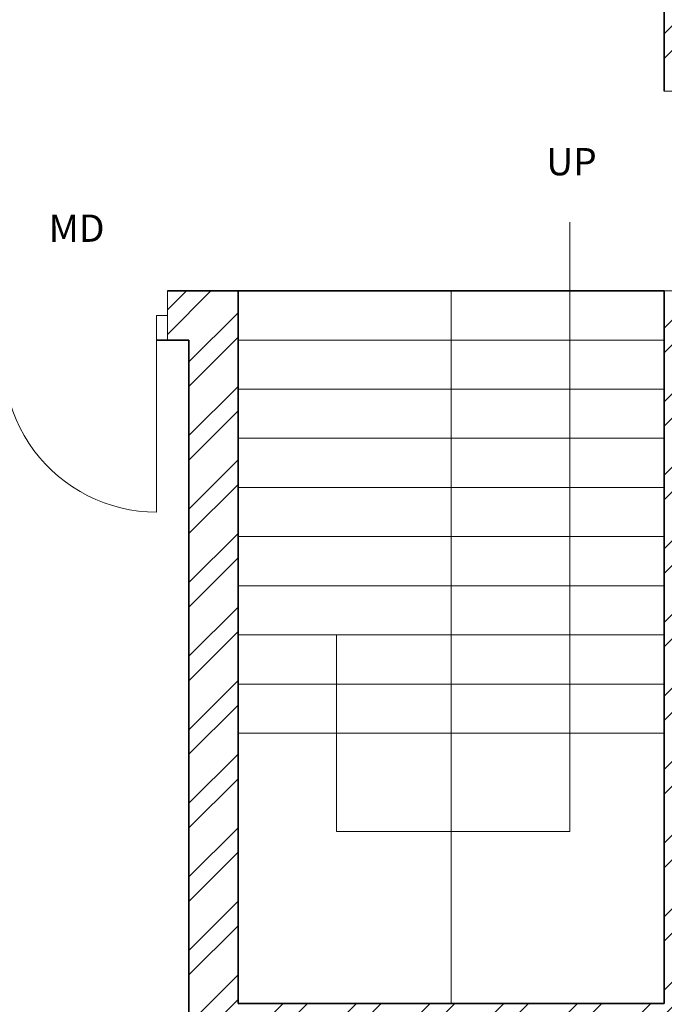
# Model space of a CAD drawing. Units: inches. Extents: x 2120 to 4013, y 1390 to 3019.
# Tile 15 of 59: x 2598 to 2716, y 1784 to 1964. Entities that reach past the tile are written whole.
import ezdxf

# ---------------------------------------------------------------- set-up
doc = ezdxf.new("R2010")
doc.units = ezdxf.units.IN
for name, color, linetype, lineweight in [('A-ANNO-TEXT', 7, 'Continuous', 18), ('A-DOOR', 3, 'Continuous', 18), ('A-FLOR-STRS', 7, 'Continuous', 18), ('A-WALL', 7, 'Continuous', 35), ('A-WALL-PATT', 252, 'Continuous', 13)]:
    doc.layers.add(name, color=color, linetype=linetype, lineweight=lineweight)
doc.styles.get("Standard").update_dxf_attribs({"font": 'arial.ttf'})

# ---------------------------------------------------------------- blocks, each defined once
blk = doc.blocks.new('DOOR-SWING-36IN-109p07DEG')
for p, q in [((9, 36.56), (0, 36.56)), ((0, 36.56), (4.5, 36.56)), ((4.5, 36.56), (4.5, 34.56)), ((9, 36.56), (9, 36.56)), ((4.5, 34.56), (40.5, 34.56)), ((4.5, 0), (4.5, 2)), ((9, 0), (0, 0)), ((0, 0), (4.5, 0))]:
    blk.add_line(p, q)
blk.add_arc((10.9, 31.1), 29.8, 257.5927, 6.6652)
blk = doc.blocks.new('DOOR-SWING-36IN-106p79DEG')
for p, q in [((0, 40.5), (0, 31.5)), ((30.74, 31.5), (30.74, 40.5)), ((30.74, 40.5), (30.74, 36)), ((0, 31.5), (0, 36)), ((0, 36), (2, 36)), ((30.74, 36), (28.74, 36)), ((28.74, 36), (28.74, 0))]:
    blk.add_line(p, q)
blk.add_arc((28.74, 27.93), 27.93, 163.2075, 270)
blk = doc.blocks.new('STAIR-DOGLEG-PLAN')
for p, q in [((60.72, 143.1), (60.72, 31.5)), ((39, 0), (39, 130.5)), ((78, 121.5), (0, 121.5)), ((78, 112.5), (0, 112.5)), ((78, 103.5), (0, 103.5)), ((78, 94.5), (0, 94.5)), ((78, 85.5), (0, 85.5)), ((78, 76.5), (0, 76.5)), ((78, 67.5), (0, 67.5)), ((18.01, 31.5), (18.01, 67.5)), ((78, 58.5), (0, 58.5)), ((78, 49.5), (0, 49.5)), ((60.72, 31.5), (18.01, 31.5)), ((60.72, 31.5), (18.01, 31.5))]:
    blk.add_line(p, q)

msp = doc.modelspace()

# ---------------------------------------------------------------- hatches: boundary and pattern name
at = {"layer": 'A-WALL-PATT'}
h = msp.add_hatch(dxfattribs=at)
h.set_pattern_fill('ANSI32', color=256)
h.paths.add_polyline_path([(2271.7331, 2343.531), (2283.3788, 2343.531), (2283.3788, 2348.031), (2283.3788, 2352.5306), (2262.7331, 2352.5306), (2262.7331, 2182.638), (2267.2331, 2182.638), (2271.7331, 2182.638), (2271.7331, 2219.031), (2391.7331, 2219.031), (2391.7331, 2214.189), (2393.9831, 2214.189), (2396.2331, 2214.189), (2396.2331, 2219.031), (2420.2331, 2219.031), (2420.2331, 2225.7535), (2417.2197, 2225.7535), (2415.7331, 2225.7535), (2415.7331, 2223.5306), (2271.7331, 2223.5306)])
h.paths.add_polyline_path([(2380.0942, 2352.5306), (2343.3788, 2352.5306), (2343.3788, 2343.531), (2363.2331, 2343.531), (2363.2331, 2288.8489), (2365.4831, 2288.8489), (2367.7331, 2288.8489), (2367.7331, 2343.531), (2380.0942, 2343.531)], flags=17)
h.paths.add_polyline_path([(2432.4339, 2352.5306), (2404.0943, 2352.5306), (2404.0943, 2343.531), (2415.7331, 2343.531), (2415.7331, 2264.0306), (2367.7331, 2264.0306), (2367.7331, 2266.4872), (2363.2331, 2266.4872), (2363.2331, 2259.531), (2367.7331, 2259.531), (2415.7331, 2259.531), (2415.7331, 2255.0658), (2420.2331, 2255.0658), (2420.2331, 2259.531), (2424.5717, 2259.531), (2424.5717, 2261.781), (2424.5717, 2264.0306), (2420.2331, 2264.0306), (2420.2331, 2343.531), (2432.4339, 2343.531)])
h.paths.add_polyline_path([(2508.9115, 2352.5306), (2456.4339, 2352.5306), (2456.4339, 2343.531), (2468.2331, 2343.531), (2468.2331, 2264.0306), (2448.0487, 2264.0306), (2448.0487, 2259.531), (2468.2331, 2259.531), (2468.2331, 2255.5496), (2472.7331, 2255.5496), (2472.7331, 2343.531), (2508.9115, 2343.531)])
h.paths.add_polyline_path([(2637.7331, 2352.5306), (2544.9116, 2352.5306), (2544.9116, 2343.531), (2589.7331, 2343.531), (2633.2331, 2343.531), (2637.7331, 2343.531)])
h.paths.add_polyline_path([(2594.2331, 2343.5306), (2589.7331, 2343.5306), (2589.7331, 2259.5306), (2589.7331, 2252.4915), (2591.9831, 2252.4915), (2594.2331, 2252.4915)])
h.paths.add_polyline_path([(2637.7331, 2223.5306), (2594.2331, 2223.5306), (2594.2331, 2230.1988), (2591.9831, 2230.1988), (2589.7331, 2230.1988), (2589.7331, 2223.5306), (2472.7331, 2223.5306), (2468.2331, 2223.5306), (2468.2331, 2219.031), (2628.7331, 2219.031), (2628.7331, 2138.031), (2637.7331, 2138.031)])
h.paths.add_polyline_path([(3822.6535, 2458.4402), (3874.9468, 2458.4402), (3874.9468, 2476.9866), (3822.6535, 2476.9866)], flags=9)
h.paths.add_polyline_path([(3834.6921, 2781.8174), (3935.9206, 2781.8174), (3935.9206, 2800.3638), (3834.6921, 2800.3638)], flags=9)
h.paths.add_polyline_path([(3832.2843, 2837.9683), (3884.5776, 2837.9683), (3884.5776, 2856.5146), (3832.2843, 2856.5146)], flags=9)
h.paths.add_polyline_path([(3830.9388, 2861.4782), (3956.8958, 2861.4782), (3956.8958, 2880.0245), (3830.9388, 2880.0245)], flags=9)
h.paths.add_polyline_path([(3870.6966, 2352.5752), (3887.9272, 2352.5752), (3887.9272, 2377.3037), (3870.6966, 2377.3037)], flags=9)
h.paths.add_polyline_path([(3289.2701, 2413.161), (3435.2223, 2413.161), (3435.2223, 2450.2538), (3289.2701, 2450.2538)], flags=9)
h.paths.add_polyline_path([(2487.6944, 2414.3601), (2637.8335, 2414.3601), (2637.8335, 2451.4528), (2487.6944, 2451.4528)], flags=9)
h.paths.add_polyline_path([(2567.3724, 1457.9199), (2815.296, 1457.9199), (2815.296, 1495.0127), (2567.3724, 1495.0127)], flags=9)
h.paths.add_polyline_path([(2655.3825, 2093.2363), (2685.9555, 2093.2363), (2685.9555, 2111.8937), (2655.3825, 2111.8937)], flags=9)
h.paths.add_polyline_path([(2543.9218, 1550.6671), (2587.8406, 1550.6671), (2587.8406, 1569.3244), (2543.9218, 1569.3244)], flags=9)
h.paths.add_polyline_path([(2905.1384, 1543.8113), (2949.0572, 1543.8113), (2949.0572, 1562.4686), (2905.1384, 1562.4686)], flags=9)
h.paths.add_polyline_path([(2736.4118, 1702.4736), (2784.2153, 1702.4736), (2784.2153, 1721.1309), (2736.4118, 1721.1309)], flags=9)
h.paths.add_polyline_path([(2912.8666, 1710.4168), (2951.707, 1710.4168), (2951.707, 1729.0741), (2912.8666, 1729.0741)], flags=9)
h.paths.add_polyline_path([(2923.5785, 1763.5038), (2959.7279, 1763.5038), (2959.7279, 1782.1611), (2923.5785, 1782.1611)], flags=9)
h.paths.add_polyline_path([(2925.2114, 1809.6137), (2967.1861, 1809.6137), (2967.1861, 1828.271), (2925.2114, 1828.271)], flags=9)
h.paths.add_polyline_path([(2996.2711, 1878.9003), (2996.2711, 1913.109), (2977.6138, 1913.109), (2977.6138, 1878.9003)], flags=9)
h.paths.add_polyline_path([(2883.0859, 1895.7192), (2927.1855, 1895.7192), (2927.1855, 1914.3766), (2883.0859, 1914.3766)], flags=9)
h.paths.add_polyline_path([(2787.3924, 1810.8013), (2841.0213, 1810.8013), (2841.0213, 1829.4587), (2787.3924, 1829.4587)], flags=9)
h.paths.add_polyline_path([(2775.6399, 2101.7395), (2829.2689, 2101.7395), (2829.2689, 2120.3968), (2775.6399, 2120.3968)], flags=9)
h.paths.add_polyline_path([(2913.0263, 2075.817), (2951.8667, 2075.817), (2951.8667, 2094.4744), (2913.0263, 2094.4744)], flags=9)
h.paths.add_polyline_path([(2929.966, 2133.3669), (2966.1154, 2133.3669), (2966.1154, 2152.0243), (2929.966, 2152.0243)], flags=9)
h.paths.add_polyline_path([(2932.7502, 2182.6088), (2968.8996, 2182.6088), (2968.8996, 2201.2662), (2932.7502, 2201.2662)], flags=9)
h.paths.add_polyline_path([(2996.0681, 2266.3173), (2996.0681, 2300.5261), (2977.4108, 2300.5261), (2977.4108, 2266.3173)], flags=9)
h.paths.add_polyline_path([(2885.1039, 2279.2186), (2929.2035, 2279.2186), (2929.2035, 2297.8759), (2885.1039, 2297.8759)], flags=9)
h.paths.add_polyline_path([(2735.7042, 2218.3197), (2783.5078, 2218.3197), (2783.5078, 2236.9771), (2735.7042, 2236.9771)], flags=9)
h.paths.add_polyline_path([(2635.6049, 2044.0085), (2648.9678, 2044.0085), (2648.9678, 2054.312), (2635.6049, 2054.312)], flags=9)
h.paths.add_polyline_path([(2714.0148, 1923.0473), (2727.3777, 1923.0473), (2727.3777, 1933.3508), (2714.0148, 1933.3508)], flags=9)
h.paths.add_polyline_path([(2709.0345, 1988.1628), (2722.3974, 1988.1628), (2722.3974, 1998.4663), (2709.0345, 1998.4663)], flags=9)
h.paths.add_polyline_path([(2592.8935, 1962.1763), (2606.2564, 1962.1763), (2606.2564, 1972.4799), (2592.8935, 1972.4799)], flags=9)
h.paths.add_polyline_path([(2618.3996, 1985.9724), (2644.1942, 1985.9724), (2644.1942, 1996.2759), (2618.3996, 1996.2759)], flags=9)
h.paths.add_polyline_path([(2601.279, 1920.5869), (2614.6419, 1920.5869), (2614.6419, 1930.8904), (2601.279, 1930.8904)], flags=9)
h.paths.add_polyline_path([(2692.3278, 1932.7645), (2704.5311, 1932.7645), (2704.5311, 1943.0681), (2692.3278, 1943.0681)], flags=9)
h.paths.add_polyline_path([(2311.122, 1672.7318), (2355.0408, 1672.7318), (2355.0408, 1691.3892), (2311.122, 1691.3892)], flags=9)
h.paths.add_polyline_path([(2456.2551, 1632.3198), (2492.4796, 1632.3198), (2492.4796, 1650.9772), (2456.2551, 1650.9772)], flags=9)
h.paths.add_polyline_path([(2401.0766, 1631.4793), (2437.301, 1631.4793), (2437.301, 1650.1367), (2401.0766, 1650.1367)], flags=9)
h.paths.add_polyline_path([(2546.7054, 1700.9235), (2594.509, 1700.9235), (2594.509, 1719.5809), (2546.7054, 1719.5809)], flags=9)
h.paths.add_polyline_path([(2445.4866, 1766.9937), (2497.5261, 1766.9937), (2497.5261, 1785.651), (2445.4866, 1785.651)], flags=9)
h.paths.add_polyline_path([(2287.9992, 1739.7675), (2326.8396, 1739.7675), (2326.8396, 1758.4248), (2287.9992, 1758.4248)], flags=9)
h.paths.add_polyline_path([(2458.5279, 1924.7607), (2510.5675, 1924.7607), (2510.5675, 1943.4181), (2458.5279, 1943.4181)], flags=9)
h.paths.add_polyline_path([(2309.2811, 1902.7642), (2345.4305, 1902.7642), (2345.4305, 1921.4215), (2309.2811, 1921.4215)], flags=9)
h.paths.add_polyline_path([(2490.7554, 2018.9392), (2530.7896, 2018.9392), (2530.7896, 2037.5965), (2490.7554, 2037.5965)], flags=9)
h.paths.add_polyline_path([(2402.143, 2024.7393), (2438.5414, 2024.7393), (2438.5414, 2043.3966), (2402.143, 2043.3966)], flags=9)
h.paths.add_polyline_path([(2287.856, 1931.7926), (2326.6964, 1931.7926), (2326.6964, 1950.4499), (2287.856, 1950.4499)], flags=9)
h.paths.add_polyline_path([(2281.7979, 2193.5771), (2320.6383, 2193.5771), (2320.6383, 2212.2344), (2281.7979, 2212.2344)], flags=25)
h.paths.add_polyline_path([(2484.0754, 2093.892), (2536.115, 2093.892), (2536.115, 2112.5494), (2484.0754, 2112.5494)], flags=9)
h.paths.add_polyline_path([(2624.7948, 2281.8639), (2624.7948, 2311.4137), (2606.1375, 2311.4137), (2606.1375, 2281.8639)], flags=9)
h.paths.add_polyline_path([(2507.5036, 2290.3639), (2541.934, 2290.3639), (2541.934, 2309.0212), (2507.5036, 2309.0212)], flags=9)
h.paths.add_polyline_path([(2423.1076, 2285.2202), (2459.332, 2285.2202), (2459.332, 2303.8776), (2423.1076, 2303.8776)], flags=9)
h.paths.add_polyline_path([(2374.5467, 2289.6272), (2410.7711, 2289.6272), (2410.7711, 2308.2846), (2374.5467, 2308.2846)], flags=25)
h.paths.add_polyline_path([(2277.4907, 2227.5651), (2316.3311, 2227.5651), (2316.3311, 2246.2224), (2277.4907, 2246.2224)], flags=25)
h.paths.add_polyline_path([(2655.3825, 2093.2367), (2685.9555, 2093.2367), (2685.9555, 2111.894), (2655.3825, 2111.894)], flags=9)
h.paths.add_polyline_path([(2543.9217, 1550.6674), (2587.8406, 1550.6674), (2587.8406, 1569.3247), (2543.9217, 1569.3247)], flags=9)
h.paths.add_polyline_path([(2905.1384, 1543.8116), (2949.0572, 1543.8116), (2949.0572, 1562.4689), (2905.1384, 1562.4689)], flags=9)
h.paths.add_polyline_path([(2736.4118, 1702.4739), (2784.2153, 1702.4739), (2784.2153, 1721.1312), (2736.4118, 1721.1312)], flags=9)
h.paths.add_polyline_path([(2912.8666, 1710.4171), (2951.707, 1710.4171), (2951.707, 1729.0744), (2912.8666, 1729.0744)], flags=9)
h.paths.add_polyline_path([(2923.5785, 1763.5041), (2959.7279, 1763.5041), (2959.7279, 1782.1614), (2923.5785, 1782.1614)], flags=9)
h.paths.add_polyline_path([(2925.2114, 1809.614), (2967.1861, 1809.614), (2967.1861, 1828.2713), (2925.2114, 1828.2713)], flags=9)
h.paths.add_polyline_path([(2996.2711, 1878.9006), (2996.2711, 1913.1094), (2977.6137, 1913.1094), (2977.6137, 1878.9006)], flags=9)
h.paths.add_polyline_path([(2883.0859, 1895.7195), (2927.1855, 1895.7195), (2927.1855, 1914.3769), (2883.0859, 1914.3769)], flags=9)
h.paths.add_polyline_path([(2787.3924, 1810.8016), (2841.0213, 1810.8016), (2841.0213, 1829.459), (2787.3924, 1829.459)], flags=9)
h.paths.add_polyline_path([(2775.6399, 2101.7398), (2829.2688, 2101.7398), (2829.2688, 2120.3971), (2775.6399, 2120.3971)], flags=9)
h.paths.add_polyline_path([(2913.0263, 2075.8173), (2951.8667, 2075.8173), (2951.8667, 2094.4747), (2913.0263, 2094.4747)], flags=9)
h.paths.add_polyline_path([(2929.966, 2133.3672), (2966.1154, 2133.3672), (2966.1154, 2152.0246), (2929.966, 2152.0246)], flags=9)
h.paths.add_polyline_path([(2932.7502, 2182.6091), (2968.8996, 2182.6091), (2968.8996, 2201.2665), (2932.7502, 2201.2665)], flags=9)
h.paths.add_polyline_path([(2996.0681, 2266.3176), (2996.0681, 2300.5264), (2977.4108, 2300.5264), (2977.4108, 2266.3176)], flags=9)
h.paths.add_polyline_path([(2885.1039, 2279.2189), (2929.2035, 2279.2189), (2929.2035, 2297.8762), (2885.1039, 2297.8762)], flags=9)
h.paths.add_polyline_path([(2735.7042, 2218.32), (2783.5078, 2218.32), (2783.5078, 2236.9774), (2735.7042, 2236.9774)], flags=9)
h.paths.add_polyline_path([(2635.6048, 2044.0088), (2648.9677, 2044.0088), (2648.9677, 2054.3123), (2635.6048, 2054.3123)], flags=9)
h.paths.add_polyline_path([(2714.0148, 1923.0476), (2727.3777, 1923.0476), (2727.3777, 1933.3511), (2714.0148, 1933.3511)], flags=9)
h.paths.add_polyline_path([(2709.0345, 1988.1631), (2722.3974, 1988.1631), (2722.3974, 1998.4666), (2709.0345, 1998.4666)], flags=9)
h.paths.add_polyline_path([(2592.8935, 1962.1766), (2606.2564, 1962.1766), (2606.2564, 1972.4802), (2592.8935, 1972.4802)], flags=9)
h.paths.add_polyline_path([(2618.3995, 1985.9727), (2644.1942, 1985.9727), (2644.1942, 1996.2762), (2618.3995, 1996.2762)], flags=9)
h.paths.add_polyline_path([(2601.279, 1920.5872), (2614.6419, 1920.5872), (2614.6419, 1930.8908), (2601.279, 1930.8908)], flags=9)
h.paths.add_polyline_path([(2692.3278, 1932.7648), (2704.5311, 1932.7648), (2704.5311, 1943.0684), (2692.3278, 1943.0684)], flags=9)
h.paths.add_polyline_path([(2311.122, 1672.7321), (2355.0408, 1672.7321), (2355.0408, 1691.3895), (2311.122, 1691.3895)], flags=9)
h.paths.add_polyline_path([(2456.2551, 1632.3201), (2492.4795, 1632.3201), (2492.4795, 1650.9775), (2456.2551, 1650.9775)], flags=9)
h.paths.add_polyline_path([(2401.0766, 1631.4796), (2437.301, 1631.4796), (2437.301, 1650.137), (2401.0766, 1650.137)], flags=9)
h.paths.add_polyline_path([(2546.7054, 1700.9238), (2594.509, 1700.9238), (2594.509, 1719.5812), (2546.7054, 1719.5812)], flags=9)
h.paths.add_polyline_path([(2445.4866, 1766.994), (2497.5261, 1766.994), (2497.5261, 1785.6513), (2445.4866, 1785.6513)], flags=9)
h.paths.add_polyline_path([(2287.9992, 1739.7678), (2326.8396, 1739.7678), (2326.8396, 1758.4251), (2287.9992, 1758.4251)], flags=9)
h.paths.add_polyline_path([(2458.5279, 1924.7611), (2510.5675, 1924.7611), (2510.5675, 1943.4184), (2458.5279, 1943.4184)], flags=9)
h.paths.add_polyline_path([(2309.2811, 1902.7645), (2345.4305, 1902.7645), (2345.4305, 1921.4218), (2309.2811, 1921.4218)], flags=9)
h.paths.add_polyline_path([(2490.7554, 2018.9395), (2530.7895, 2018.9395), (2530.7895, 2037.5968), (2490.7554, 2037.5968)], flags=9)
h.paths.add_polyline_path([(2402.143, 2024.7396), (2438.5413, 2024.7396), (2438.5413, 2043.3969), (2402.143, 2043.3969)], flags=9)
h.paths.add_polyline_path([(2287.856, 1931.7929), (2326.6964, 1931.7929), (2326.6964, 1950.4502), (2287.856, 1950.4502)], flags=9)
h.paths.add_polyline_path([(2281.7979, 2193.5774), (2320.6383, 2193.5774), (2320.6383, 2212.2347), (2281.7979, 2212.2347)], flags=25)
h.paths.add_polyline_path([(2484.0754, 2093.8924), (2536.115, 2093.8924), (2536.115, 2112.5497), (2484.0754, 2112.5497)], flags=9)
h.paths.add_polyline_path([(2624.7948, 2281.8642), (2624.7948, 2311.414), (2606.1374, 2311.414), (2606.1374, 2281.8642)], flags=9)
h.paths.add_polyline_path([(2507.5035, 2290.3642), (2541.934, 2290.3642), (2541.934, 2309.0215), (2507.5035, 2309.0215)], flags=9)
h.paths.add_polyline_path([(2423.1075, 2285.2205), (2459.332, 2285.2205), (2459.332, 2303.8779), (2423.1075, 2303.8779)], flags=9)
h.paths.add_polyline_path([(2374.5467, 2289.6275), (2410.7711, 2289.6275), (2410.7711, 2308.2849), (2374.5467, 2308.2849)], flags=25)
h.paths.add_polyline_path([(2277.4907, 2227.5654), (2316.3311, 2227.5654), (2316.3311, 2246.2227), (2277.4907, 2246.2227)], flags=25)
h = msp.add_hatch(dxfattribs=at)
h.set_pattern_fill('ANSI32', color=256)
h.paths.add_polyline_path([(2271.7331, 1980.389), (2262.7331, 1980.389), (2262.7331, 1912.8434), (2267.2331, 1912.8434), (2271.7331, 1912.8434), (2271.7331, 1922.531), (2351.2331, 1922.531), (2351.2331, 1901.4728), (2355.7331, 1901.4728), (2355.7331, 1922.531), (2357.9815, 1922.531), (2357.9815, 1926.5306), (2271.7331, 1926.5306)])
h.paths.add_polyline_path([(2589.2331, 1949.1622), (2584.7331, 1949.1622), (2580.2331, 1949.1622), (2580.2331, 1874.5306), (2355.7331, 1874.5306), (2355.7331, 1880.1922), (2351.2331, 1880.1922), (2351.2331, 1874.5306), (2271.7331, 1874.5306), (2271.7331, 1888.8431), (2262.7331, 1888.8431), (2262.7331, 1842.2909), (2267.2331, 1842.2909), (2271.7331, 1842.2909), (2271.7331, 1865.531), (2415.7331, 1865.531), (2415.7331, 1779.7286), (2420.2331, 1779.7286), (2420.2331, 1865.531), (2589.2331, 1865.531)])
h.paths.add_polyline_path([(2271.7331, 1782.2906), (2262.7331, 1782.2906), (2262.7331, 1711.4639), (2267.2331, 1711.4639), (2271.7331, 1711.4639), (2271.7331, 1738.031), (2420.2331, 1738.031), (2420.2331, 1742.531), (2420.2331, 1747.3376), (2417.9831, 1747.3376), (2415.7331, 1747.3376), (2415.7331, 1742.5306), (2271.7331, 1742.5306)])
h.paths.add_polyline_path([(2271.7331, 1627.031), (2362.3957, 1627.031), (2362.3957, 1629.281), (2362.3957, 1631.5306), (2271.7331, 1631.5306), (2271.7331, 1675.4636), (2262.7331, 1675.4636), (2262.7331, 1581.531), (2405.3032, 1581.531), (2405.3032, 1586.031), (2405.3032, 1590.5306), (2396.2331, 1590.5306), (2396.2331, 1691.4513), (2418.7206, 1691.4513), (2418.7206, 1695.951), (2396.2331, 1695.951), (2391.7331, 1695.951), (2391.7331, 1631.5306), (2386.7425, 1631.5306), (2386.7425, 1629.2806), (2386.7425, 1627.031), (2391.7331, 1627.031), (2391.7331, 1586.1709), (2271.7331, 1586.1709)])
h.paths.add_polyline_path([(2459.6703, 1590.5306), (2429.3032, 1590.5306), (2429.3032, 1581.531), (2459.6703, 1581.531), (2459.6703, 1586.031)])
h.paths.add_polyline_path([(2501.2331, 1590.531), (2501.2331, 1665.0195), (2498.9831, 1665.0195), (2496.7331, 1665.0195), (2496.7331, 1590.5306), (2483.8201, 1590.5306), (2483.8201, 1590.1579), (2483.6704, 1590.1579), (2483.6704, 1581.531), (2505.0196, 1581.531), (2505.0196, 1583.781), (2505.0196, 1586.0306), (2501.2331, 1586.0306)])
h.paths.add_polyline_path([(2544.1361, 1583.781), (2544.1361, 1586.0306), (2527.1368, 1586.0306), (2527.1368, 1583.7806), (2527.1368, 1581.531), (2544.1361, 1581.531)])
h.paths.add_polyline_path([(3822.6535, 2458.4402), (3874.9468, 2458.4402), (3874.9468, 2476.9866), (3822.6535, 2476.9866)], flags=9)
h.paths.add_polyline_path([(3834.6921, 2781.8174), (3935.9206, 2781.8174), (3935.9206, 2800.3638), (3834.6921, 2800.3638)], flags=9)
h.paths.add_polyline_path([(3832.2843, 2837.9683), (3884.5776, 2837.9683), (3884.5776, 2856.5146), (3832.2843, 2856.5146)], flags=9)
h.paths.add_polyline_path([(3830.9388, 2861.4782), (3956.8958, 2861.4782), (3956.8958, 2880.0245), (3830.9388, 2880.0245)], flags=9)
h.paths.add_polyline_path([(3870.6966, 2352.5752), (3887.9272, 2352.5752), (3887.9272, 2377.3037), (3870.6966, 2377.3037)], flags=9)
h.paths.add_polyline_path([(3289.2701, 2413.161), (3435.2223, 2413.161), (3435.2223, 2450.2538), (3289.2701, 2450.2538)], flags=9)
h.paths.add_polyline_path([(2487.6944, 2414.3601), (2637.8335, 2414.3601), (2637.8335, 2451.4528), (2487.6944, 2451.4528)], flags=9)
h.paths.add_polyline_path([(2567.3724, 1457.9199), (2815.296, 1457.9199), (2815.296, 1495.0127), (2567.3724, 1495.0127)], flags=9)
h.paths.add_polyline_path([(2655.3825, 2093.2363), (2685.9555, 2093.2363), (2685.9555, 2111.8937), (2655.3825, 2111.8937)], flags=9)
h.paths.add_polyline_path([(2543.9218, 1550.6671), (2587.8406, 1550.6671), (2587.8406, 1569.3244), (2543.9218, 1569.3244)], flags=9)
h.paths.add_polyline_path([(2905.1384, 1543.8113), (2949.0572, 1543.8113), (2949.0572, 1562.4686), (2905.1384, 1562.4686)], flags=9)
h.paths.add_polyline_path([(2736.4118, 1702.4736), (2784.2153, 1702.4736), (2784.2153, 1721.1309), (2736.4118, 1721.1309)], flags=9)
h.paths.add_polyline_path([(2912.8666, 1710.4168), (2951.707, 1710.4168), (2951.707, 1729.0741), (2912.8666, 1729.0741)], flags=9)
h.paths.add_polyline_path([(2923.5785, 1763.5038), (2959.7279, 1763.5038), (2959.7279, 1782.1611), (2923.5785, 1782.1611)], flags=9)
h.paths.add_polyline_path([(2925.2114, 1809.6137), (2967.1861, 1809.6137), (2967.1861, 1828.271), (2925.2114, 1828.271)], flags=9)
h.paths.add_polyline_path([(2996.2711, 1878.9003), (2996.2711, 1913.109), (2977.6138, 1913.109), (2977.6138, 1878.9003)], flags=9)
h.paths.add_polyline_path([(2883.0859, 1895.7192), (2927.1855, 1895.7192), (2927.1855, 1914.3766), (2883.0859, 1914.3766)], flags=9)
h.paths.add_polyline_path([(2787.3924, 1810.8013), (2841.0213, 1810.8013), (2841.0213, 1829.4587), (2787.3924, 1829.4587)], flags=9)
h.paths.add_polyline_path([(2775.6399, 2101.7395), (2829.2689, 2101.7395), (2829.2689, 2120.3968), (2775.6399, 2120.3968)], flags=9)
h.paths.add_polyline_path([(2913.0263, 2075.817), (2951.8667, 2075.817), (2951.8667, 2094.4744), (2913.0263, 2094.4744)], flags=9)
h.paths.add_polyline_path([(2929.966, 2133.3669), (2966.1154, 2133.3669), (2966.1154, 2152.0243), (2929.966, 2152.0243)], flags=9)
h.paths.add_polyline_path([(2932.7502, 2182.6088), (2968.8996, 2182.6088), (2968.8996, 2201.2662), (2932.7502, 2201.2662)], flags=9)
h.paths.add_polyline_path([(2996.0681, 2266.3173), (2996.0681, 2300.5261), (2977.4108, 2300.5261), (2977.4108, 2266.3173)], flags=9)
h.paths.add_polyline_path([(2885.1039, 2279.2186), (2929.2035, 2279.2186), (2929.2035, 2297.8759), (2885.1039, 2297.8759)], flags=9)
h.paths.add_polyline_path([(2735.7042, 2218.3197), (2783.5078, 2218.3197), (2783.5078, 2236.9771), (2735.7042, 2236.9771)], flags=9)
h.paths.add_polyline_path([(2635.6049, 2044.0085), (2648.9678, 2044.0085), (2648.9678, 2054.312), (2635.6049, 2054.312)], flags=9)
h.paths.add_polyline_path([(2714.0148, 1923.0473), (2727.3777, 1923.0473), (2727.3777, 1933.3508), (2714.0148, 1933.3508)], flags=9)
h.paths.add_polyline_path([(2709.0345, 1988.1628), (2722.3974, 1988.1628), (2722.3974, 1998.4663), (2709.0345, 1998.4663)], flags=9)
h.paths.add_polyline_path([(2592.8935, 1962.1763), (2606.2564, 1962.1763), (2606.2564, 1972.4799), (2592.8935, 1972.4799)], flags=9)
h.paths.add_polyline_path([(2618.3996, 1985.9724), (2644.1942, 1985.9724), (2644.1942, 1996.2759), (2618.3996, 1996.2759)], flags=9)
h.paths.add_polyline_path([(2601.279, 1920.5869), (2614.6419, 1920.5869), (2614.6419, 1930.8904), (2601.279, 1930.8904)], flags=9)
h.paths.add_polyline_path([(2692.3278, 1932.7645), (2704.5311, 1932.7645), (2704.5311, 1943.0681), (2692.3278, 1943.0681)], flags=9)
h.paths.add_polyline_path([(2311.122, 1672.7318), (2355.0408, 1672.7318), (2355.0408, 1691.3892), (2311.122, 1691.3892)], flags=25)
h.paths.add_polyline_path([(2456.2551, 1632.3198), (2492.4796, 1632.3198), (2492.4796, 1650.9772), (2456.2551, 1650.9772)], flags=9)
h.paths.add_polyline_path([(2401.0766, 1631.4793), (2437.301, 1631.4793), (2437.301, 1650.1367), (2401.0766, 1650.1367)], flags=9)
h.paths.add_polyline_path([(2546.7054, 1700.9235), (2594.509, 1700.9235), (2594.509, 1719.5809), (2546.7054, 1719.5809)], flags=9)
h.paths.add_polyline_path([(2445.4866, 1766.9937), (2497.5261, 1766.9937), (2497.5261, 1785.651), (2445.4866, 1785.651)], flags=9)
h.paths.add_polyline_path([(2287.9992, 1739.7675), (2326.8396, 1739.7675), (2326.8396, 1758.4248), (2287.9992, 1758.4248)], flags=24)
h.paths.add_polyline_path([(2458.5279, 1924.7607), (2510.5675, 1924.7607), (2510.5675, 1943.4181), (2458.5279, 1943.4181)], flags=25)
h.paths.add_polyline_path([(2309.2811, 1902.7642), (2345.4305, 1902.7642), (2345.4305, 1921.4215), (2309.2811, 1921.4215)], flags=25)
h.paths.add_polyline_path([(2490.7554, 2018.9392), (2530.7896, 2018.9392), (2530.7896, 2037.5965), (2490.7554, 2037.5965)], flags=9)
h.paths.add_polyline_path([(2402.143, 2024.7393), (2438.5414, 2024.7393), (2438.5414, 2043.3966), (2402.143, 2043.3966)], flags=9)
h.paths.add_polyline_path([(2287.856, 1931.7926), (2326.6964, 1931.7926), (2326.6964, 1950.4499), (2287.856, 1950.4499)], flags=25)
h.paths.add_polyline_path([(2281.7979, 2193.5771), (2320.6383, 2193.5771), (2320.6383, 2212.2344), (2281.7979, 2212.2344)], flags=9)
h.paths.add_polyline_path([(2484.0754, 2093.892), (2536.115, 2093.892), (2536.115, 2112.5494), (2484.0754, 2112.5494)], flags=9)
h.paths.add_polyline_path([(2624.7948, 2281.8639), (2624.7948, 2311.4137), (2606.1375, 2311.4137), (2606.1375, 2281.8639)], flags=9)
h.paths.add_polyline_path([(2507.5036, 2290.3639), (2541.934, 2290.3639), (2541.934, 2309.0212), (2507.5036, 2309.0212)], flags=9)
h.paths.add_polyline_path([(2423.1076, 2285.2202), (2459.332, 2285.2202), (2459.332, 2303.8776), (2423.1076, 2303.8776)], flags=9)
h.paths.add_polyline_path([(2374.5467, 2289.6272), (2410.7711, 2289.6272), (2410.7711, 2308.2846), (2374.5467, 2308.2846)], flags=9)
h.paths.add_polyline_path([(2277.4907, 2227.5651), (2316.3311, 2227.5651), (2316.3311, 2246.2224), (2277.4907, 2246.2224)], flags=9)
h.paths.add_polyline_path([(2655.3825, 2093.2367), (2685.9555, 2093.2367), (2685.9555, 2111.894), (2655.3825, 2111.894)], flags=9)
h.paths.add_polyline_path([(2543.9217, 1550.6674), (2587.8406, 1550.6674), (2587.8406, 1569.3247), (2543.9217, 1569.3247)], flags=9)
h.paths.add_polyline_path([(2905.1384, 1543.8116), (2949.0572, 1543.8116), (2949.0572, 1562.4689), (2905.1384, 1562.4689)], flags=9)
h.paths.add_polyline_path([(2736.4118, 1702.4739), (2784.2153, 1702.4739), (2784.2153, 1721.1312), (2736.4118, 1721.1312)], flags=9)
h.paths.add_polyline_path([(2912.8666, 1710.4171), (2951.707, 1710.4171), (2951.707, 1729.0744), (2912.8666, 1729.0744)], flags=9)
h.paths.add_polyline_path([(2923.5785, 1763.5041), (2959.7279, 1763.5041), (2959.7279, 1782.1614), (2923.5785, 1782.1614)], flags=9)
h.paths.add_polyline_path([(2925.2114, 1809.614), (2967.1861, 1809.614), (2967.1861, 1828.2713), (2925.2114, 1828.2713)], flags=9)
h.paths.add_polyline_path([(2996.2711, 1878.9006), (2996.2711, 1913.1094), (2977.6137, 1913.1094), (2977.6137, 1878.9006)], flags=9)
h.paths.add_polyline_path([(2883.0859, 1895.7195), (2927.1855, 1895.7195), (2927.1855, 1914.3769), (2883.0859, 1914.3769)], flags=9)
h.paths.add_polyline_path([(2787.3924, 1810.8016), (2841.0213, 1810.8016), (2841.0213, 1829.459), (2787.3924, 1829.459)], flags=9)
h.paths.add_polyline_path([(2775.6399, 2101.7398), (2829.2688, 2101.7398), (2829.2688, 2120.3971), (2775.6399, 2120.3971)], flags=9)
h.paths.add_polyline_path([(2913.0263, 2075.8173), (2951.8667, 2075.8173), (2951.8667, 2094.4747), (2913.0263, 2094.4747)], flags=9)
h.paths.add_polyline_path([(2929.966, 2133.3672), (2966.1154, 2133.3672), (2966.1154, 2152.0246), (2929.966, 2152.0246)], flags=9)
h.paths.add_polyline_path([(2932.7502, 2182.6091), (2968.8996, 2182.6091), (2968.8996, 2201.2665), (2932.7502, 2201.2665)], flags=9)
h.paths.add_polyline_path([(2996.0681, 2266.3176), (2996.0681, 2300.5264), (2977.4108, 2300.5264), (2977.4108, 2266.3176)], flags=9)
h.paths.add_polyline_path([(2885.1039, 2279.2189), (2929.2035, 2279.2189), (2929.2035, 2297.8762), (2885.1039, 2297.8762)], flags=9)
h.paths.add_polyline_path([(2735.7042, 2218.32), (2783.5078, 2218.32), (2783.5078, 2236.9774), (2735.7042, 2236.9774)], flags=9)
h.paths.add_polyline_path([(2635.6048, 2044.0088), (2648.9677, 2044.0088), (2648.9677, 2054.3123), (2635.6048, 2054.3123)], flags=9)
h.paths.add_polyline_path([(2714.0148, 1923.0476), (2727.3777, 1923.0476), (2727.3777, 1933.3511), (2714.0148, 1933.3511)], flags=9)
h.paths.add_polyline_path([(2709.0345, 1988.1631), (2722.3974, 1988.1631), (2722.3974, 1998.4666), (2709.0345, 1998.4666)], flags=9)
h.paths.add_polyline_path([(2592.8935, 1962.1766), (2606.2564, 1962.1766), (2606.2564, 1972.4802), (2592.8935, 1972.4802)], flags=9)
h.paths.add_polyline_path([(2618.3995, 1985.9727), (2644.1942, 1985.9727), (2644.1942, 1996.2762), (2618.3995, 1996.2762)], flags=9)
h.paths.add_polyline_path([(2601.279, 1920.5872), (2614.6419, 1920.5872), (2614.6419, 1930.8908), (2601.279, 1930.8908)], flags=9)
h.paths.add_polyline_path([(2692.3278, 1932.7648), (2704.5311, 1932.7648), (2704.5311, 1943.0684), (2692.3278, 1943.0684)], flags=9)
h.paths.add_polyline_path([(2311.122, 1672.7321), (2355.0408, 1672.7321), (2355.0408, 1691.3895), (2311.122, 1691.3895)], flags=25)
h.paths.add_polyline_path([(2456.2551, 1632.3201), (2492.4795, 1632.3201), (2492.4795, 1650.9775), (2456.2551, 1650.9775)], flags=9)
h.paths.add_polyline_path([(2401.0766, 1631.4796), (2437.301, 1631.4796), (2437.301, 1650.137), (2401.0766, 1650.137)], flags=9)
h.paths.add_polyline_path([(2546.7054, 1700.9238), (2594.509, 1700.9238), (2594.509, 1719.5812), (2546.7054, 1719.5812)], flags=9)
h.paths.add_polyline_path([(2445.4866, 1766.994), (2497.5261, 1766.994), (2497.5261, 1785.6513), (2445.4866, 1785.6513)], flags=9)
h.paths.add_polyline_path([(2287.9992, 1739.7678), (2326.8396, 1739.7678), (2326.8396, 1758.4251), (2287.9992, 1758.4251)], flags=24)
h.paths.add_polyline_path([(2458.5279, 1924.7611), (2510.5675, 1924.7611), (2510.5675, 1943.4184), (2458.5279, 1943.4184)], flags=25)
h.paths.add_polyline_path([(2309.2811, 1902.7645), (2345.4305, 1902.7645), (2345.4305, 1921.4218), (2309.2811, 1921.4218)], flags=25)
h.paths.add_polyline_path([(2490.7554, 2018.9395), (2530.7895, 2018.9395), (2530.7895, 2037.5968), (2490.7554, 2037.5968)], flags=9)
h.paths.add_polyline_path([(2402.143, 2024.7396), (2438.5413, 2024.7396), (2438.5413, 2043.3969), (2402.143, 2043.3969)], flags=9)
h.paths.add_polyline_path([(2287.856, 1931.7929), (2326.6964, 1931.7929), (2326.6964, 1950.4502), (2287.856, 1950.4502)], flags=25)
h.paths.add_polyline_path([(2281.7979, 2193.5774), (2320.6383, 2193.5774), (2320.6383, 2212.2347), (2281.7979, 2212.2347)], flags=9)
h.paths.add_polyline_path([(2484.0754, 2093.8924), (2536.115, 2093.8924), (2536.115, 2112.5497), (2484.0754, 2112.5497)], flags=9)
h.paths.add_polyline_path([(2624.7948, 2281.8642), (2624.7948, 2311.414), (2606.1374, 2311.414), (2606.1374, 2281.8642)], flags=9)
h.paths.add_polyline_path([(2507.5035, 2290.3642), (2541.934, 2290.3642), (2541.934, 2309.0215), (2507.5035, 2309.0215)], flags=9)
h.paths.add_polyline_path([(2423.1075, 2285.2205), (2459.332, 2285.2205), (2459.332, 2303.8779), (2423.1075, 2303.8779)], flags=9)
h.paths.add_polyline_path([(2374.5467, 2289.6275), (2410.7711, 2289.6275), (2410.7711, 2308.2849), (2374.5467, 2308.2849)], flags=9)
h.paths.add_polyline_path([(2277.4907, 2227.5654), (2316.3311, 2227.5654), (2316.3311, 2246.2227), (2277.4907, 2246.2227)], flags=9)
h = msp.add_hatch(dxfattribs=at)
h.set_pattern_fill('ANSI32', color=256)
h.paths.add_polyline_path([(2271.7331, 2122.6377), (2262.7331, 2122.6377), (2262.7331, 2040.3893), (2267.2331, 2040.3893), (2271.7331, 2040.3893), (2271.7331, 2044.8856), (2271.7331, 2070.531), (2391.7331, 2070.531), (2391.7331, 1926.5306), (2388.3993, 1926.5306), (2388.3993, 1922.531), (2395.7331, 1922.531), (2395.7331, 1992.531), (2400.4511, 1992.531), (2400.4511, 1997.0306), (2395.7331, 1997.0306), (2395.7331, 2070.531), (2443.7331, 2070.531), (2443.7331, 2046.1368), (2448.2331, 2046.1368), (2448.2331, 2070.531), (2580.2331, 2070.531), (2580.2331, 1997.0306), (2492.9076, 1997.0306), (2492.9076, 1992.531), (2580.2331, 1992.531), (2580.2331, 1983.9368), (2589.2331, 1983.9368), (2589.2331, 2070.531), (2589.2331, 2075.0306), (2396.2331, 2075.0306), (2396.2331, 2184.3565), (2393.9831, 2184.3565), (2391.7331, 2184.3565), (2391.7331, 2075.0306), (2271.7331, 2075.0306)])
h.paths.add_polyline_path([(2724.7331, 2138.0306), (2628.7331, 2138.0306), (2628.7331, 2070.5306), (2628.7331, 2067.0987), (2633.2331, 2067.0987), (2637.7331, 2067.0987), (2637.7331, 2070.531), (2657.3413, 2070.531), (2657.3413, 2079.5306), (2637.7331, 2079.5306), (2637.7331, 2129.031), (2715.7331, 2129.031), (2715.7331, 2079.5306), (2698.0378, 2079.5306), (2698.0378, 2070.531), (2715.7331, 2070.531), (2715.7331, 2012.1531), (2720.2331, 2012.1531), (2724.7331, 2012.1531)])
h.paths.add_polyline_path([(2724.7331, 2213.031), (2831.3209, 2213.031), (2831.3209, 2215.281), (2831.3209, 2217.5306), (2724.7331, 2217.5306), (2724.7331, 2343.531), (2751.8755, 2343.531), (2751.8755, 2352.5306), (2715.7331, 2352.5306), (2715.7331, 2138.031), (2724.7331, 2138.031)])
h.paths.add_polyline_path([(2902.53, 2352.5306), (2811.8755, 2352.5306), (2811.8755, 2343.531), (2867.2331, 2343.531), (2867.2331, 2217.5306), (2863.6364, 2217.5306), (2863.6364, 2213.031), (2871.7331, 2213.031), (2871.7331, 2217.531), (2871.7331, 2343.531), (2902.53, 2343.531)])
h.paths.add_polyline_path([(3009.7331, 2352.5306), (2938.53, 2352.5306), (2938.53, 2343.531), (2966.2331, 2343.531), (2966.2331, 2242.3281), (2968.4831, 2242.3281), (2970.7331, 2242.3281), (2970.7331, 2343.531), (3009.7331, 2343.531)])
h.paths.add_polyline_path([(3009.7331, 2217.5306), (2970.7331, 2217.5306), (2970.7331, 2220.5422), (2968.4831, 2220.5422), (2966.2331, 2220.5422), (2966.2331, 2217.5306), (2911.7752, 2217.5306), (2907.7331, 2217.5306), (2907.7331, 2213.0306), (2907.7331, 2194.9663), (2912.2331, 2194.9663), (2912.2331, 2213.031), (2970.7331, 2213.031), (3000.7331, 2213.031), (3000.7331, 2205.523), (3009.7331, 2205.523)])
h.paths.add_polyline_path([(3009.7331, 2181.5227), (3000.7331, 2181.5227), (3000.7331, 2165.0306), (2912.2331, 2165.0306), (2912.2331, 2170.8202), (2907.7331, 2170.8202), (2907.7331, 2165.0306), (2899.5169, 2165.0306), (2899.5169, 2162.7806), (2899.5169, 2160.531), (2907.7331, 2160.531), (2907.7331, 2137.3432), (2912.2331, 2137.3432), (2912.2331, 2160.531), (3000.7331, 2160.531), (3000.7331, 2150.4993), (3009.7331, 2150.4993)])
h.paths.add_polyline_path([(3009.7331, 2126.499), (3005.2331, 2126.499), (3000.7331, 2126.499), (3000.7331, 2112.5306), (2912.2331, 2112.5306), (2912.2331, 2115.6036), (2907.7331, 2115.6036), (2907.7331, 2108.031), (3000.7331, 2108.031), (3000.7331, 2084.7256), (3009.7331, 2084.7256)], flags=17)
h.paths.add_polyline_path([(3009.7331, 1971.531), (3009.7331, 2024.7253), (3000.7331, 2024.7253), (3000.7331, 2006.4153), (3000.7331, 1971.5306), (2864.2331, 1971.5306), (2864.2331, 2160.531), (2868.0522, 2160.531), (2868.0522, 2165.0306), (2859.7331, 2165.0306), (2859.7331, 1971.5306), (2724.7331, 1971.5306), (2724.7331, 1977.7012), (2715.7331, 1977.7012), (2715.7331, 1962.5306), (2715.7331, 1950.9035), (2720.2331, 1950.9035), (2724.7331, 1950.9035), (2724.7331, 1962.531), (2855.2331, 1962.531), (2859.7331, 1962.531), (2859.7331, 1835.031), (2864.2331, 1834.8158), (2864.2331, 1962.531), (2958.7331, 1962.531), (2958.7331, 1937.0925), (2963.2331, 1937.0925), (2963.2331, 1962.531), (3000.7331, 1962.531), (3009.7331, 1962.531)])
h.paths.add_polyline_path([(2724.7331, 1728.531), (2822.7164, 1728.531), (2822.7164, 1733.0306), (2724.7331, 1733.0306), (2724.7331, 1779.3416), (2715.7331, 1779.3416), (2715.7331, 1581.531), (2753.02, 1581.531), (2753.02, 1586.031), (2753.02, 1590.5306), (2724.7331, 1590.5306)])
h.paths.add_polyline_path([(2864.2331, 1590.531), (2864.2331, 1787.031), (2868.4075, 1787.031), (2868.4075, 1791.5306), (2859.7331, 1791.5306), (2859.7331, 1739.0306), (2859.7331, 1733.0306), (2854.3125, 1733.0306), (2854.3125, 1728.531), (2859.7331, 1728.531), (2859.7331, 1590.5306), (2813.02, 1590.5306), (2813.02, 1581.531), (2868.4123, 1581.531), (2868.4123, 1583.781), (2868.4123, 1586.0306), (2864.2331, 1586.0306)])
h.paths.add_polyline_path([(3009.7331, 1754.6619), (3000.7331, 1754.6619), (3000.7331, 1739.0306), (2912.2331, 1739.0306), (2912.2331, 1742.2257), (2907.7331, 1742.2257), (2907.7331, 1739.0306), (2907.7331, 1734.531), (3000.7331, 1734.531), (3000.7331, 1590.5306), (3000.7331, 1586.0306), (2971.3921, 1586.0306), (2971.3921, 1581.531), (3009.7331, 1581.531)])
h.paths.add_polyline_path([(2911.3921, 1583.781), (2911.3921, 1586.0306), (2891.2138, 1586.0306), (2891.2138, 1581.531), (2911.3921, 1581.531)])
h.paths.add_polyline_path([(3009.7331, 1799.8422), (3000.7331, 1799.8422), (3000.7331, 1791.5306), (2912.2331, 1791.5306), (2912.2331, 1796.3264), (2909.9831, 1796.3264), (2907.7331, 1796.3264), (2907.7331, 1791.5306), (2902.7033, 1791.5306), (2902.7033, 1787.031), (2907.7331, 1787.031), (2907.7331, 1761.1622), (2912.2331, 1761.1622), (2912.2331, 1787.031), (3000.7331, 1787.031), (3000.7331, 1778.6622), (3009.7331, 1778.6622)])
h.paths.add_polyline_path([(3009.7331, 1839.5306), (2963.2331, 1839.5306), (2963.2331, 1842.8629), (2960.9831, 1842.8629), (2958.7331, 1842.8629), (2958.7331, 1839.5306), (2907.7331, 1839.5306), (2907.7331, 1814.4599), (2912.2331, 1814.4599), (2912.2331, 1835.031), (3000.7331, 1835.031), (3000.7331, 1823.8425), (3009.7331, 1823.8425), (3009.7331, 1835.031)])
h.paths.add_polyline_path([(2963.2331, 1901.0922), (2960.9831, 1901.0922), (2958.7331, 1901.0922), (2958.7331, 1862.8843), (2963.2331, 1862.8843)], flags=17)
h.paths.add_polyline_path([(2724.7331, 1891.9826), (2724.7331, 1914.3416), (2715.7331, 1914.3416), (2715.7331, 1783.8416), (2637.7331, 1783.8416), (2637.7331, 1914.3416), (2628.7331, 1914.3416), (2624.7701, 1914.3416), (2624.7701, 1909.8416), (2624.7701, 1905.3419), (2628.7331, 1905.3419), (2628.7331, 1876.9915), (2628.7331, 1779.3419), (2637.7331, 1779.3419), (2715.7331, 1779.3419), (2724.7331, 1779.3419), (2724.7331, 1835.031)])
h.paths.add_polyline_path([(2637.7331, 1731.531), (2637.7331, 1779.3416), (2628.7331, 1779.3416), (2628.7331, 1731.5306), (2589.2331, 1731.5306), (2535.9814, 1731.5306), (2496.7331, 1731.5306), (2496.7331, 1725.6876), (2498.9831, 1725.6876), (2501.2331, 1725.6876), (2501.2331, 1727.031), (2628.7331, 1727.031), (2628.7331, 1680.4203), (2628.7331, 1590.5306), (2628.7331, 1586.0306), (2604.1361, 1586.0306), (2604.1361, 1581.531), (2637.7331, 1581.531), (2637.7331, 1590.531)])

# ---------------------------------------------------------------- linework, layer by layer
at = {"layer": 'A-WALL'}
for p, q in [((2715.7331, 1977.7015), (2715.7331, 1962.531)), ((2715.7331, 1977.7012), (2715.7331, 1962.5306)), ((2715.7331, 1962.531), (2715.7331, 1962.531)), ((2715.7331, 1962.531), (2715.7331, 1950.9035)), ((2715.7331, 1962.5306), (2715.7331, 1962.5306)), ((2715.7331, 1962.5306), (2715.7331, 1950.9032)), ((2628.7331, 1914.3419), (2624.7701, 1914.3419)), ((2628.7331, 1914.3416), (2624.7701, 1914.3416)), ((2715.7331, 1914.3419), (2628.7331, 1914.3419)), ((2715.7331, 1914.3416), (2628.7331, 1914.3416)), ((2637.7331, 1914.3419), (2637.7331, 1783.8419)), ((2637.7331, 1914.3416), (2637.7331, 1783.8416)), ((2715.7331, 1914.3419), (2715.7331, 1783.8419)), ((2715.7331, 1914.3416), (2715.7331, 1783.8416)), ((2622.7701, 1905.3419), (2628.7331, 1905.3419)), ((2622.7701, 1905.3416), (2628.7331, 1905.3416)), ((2628.7331, 1905.3419), (2628.7331, 1876.9918)), ((2628.7331, 1905.3416), (2628.7331, 1876.9915)), ((2628.7331, 1731.531), (2628.7331, 1876.9918)), ((2628.7331, 1731.5306), (2628.7331, 1876.9915)), ((2637.7331, 1783.8419), (2715.7331, 1783.8419)), ((2637.7331, 1783.8416), (2715.7331, 1783.8416))]:
    msp.add_line(p, q, dxfattribs=at)

# ---------------------------------------------------------------- block references
at = {"layer": 'A-DOOR'}
for name, p in [('DOOR-SWING-36IN-109p07DEG', (2715.7331, 1914.3419)), ('DOOR-SWING-36IN-109p07DEG', (2715.7331, 1914.3416)), ('DOOR-SWING-36IN-106p79DEG', (2594.0305, 1873.8419)), ('DOOR-SWING-36IN-106p79DEG', (2594.0305, 1873.8416))]:
    msp.add_blockref(name, p, dxfattribs=at)
at = {"layer": 'A-FLOR-STRS'}
for p in [(2637.7331, 1783.8419), (2637.7331, 1783.8416)]:
    msp.add_blockref('STAIR-DOGLEG-PLAN', p, dxfattribs=at)

# ---------------------------------------------------------------- texts
at = {"layer": 'A-ANNO-TEXT', "char_height": 5, "attachment_point": 1}
for s, width, insert in [('UP', 26.183597, (2694.1269, 1940.4951)), ('UP', 26.183597, (2694.1269, 1940.4948)), ('MD', 56.213303, (2603.0474, 1928.3174)), ('MD', 56.213303, (2603.0474, 1928.3171))]:
    msp.add_mtext_dynamic_manual_height_columns(s, width=width, gutter_width=12.5, heights=[0], dxfattribs=dict(at, insert=insert))

doc.saveas('drawing.dxf')
